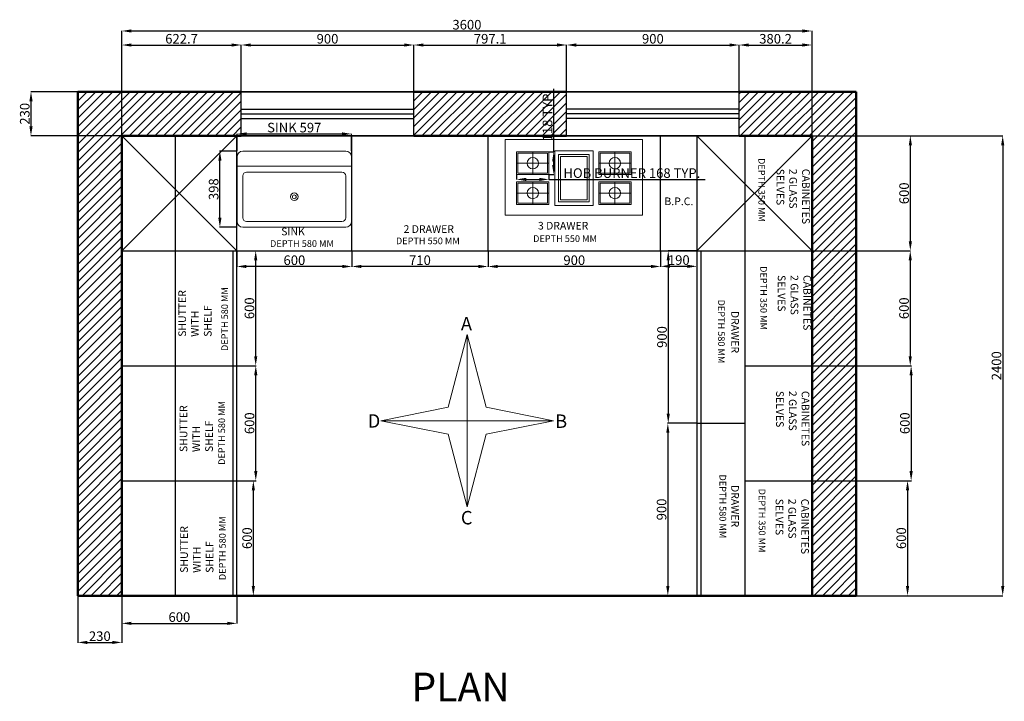
# Model space of a CAD drawing. Units: millimetres. Extents: x 4283 to 9420, y -2853 to 5191.
# Tile 2 of 2: x 4283 to 9420, y 1633 to 5191. Entities that reach past the tile are written whole.
import ezdxf

# ---------------------------------------------------------------- set-up
doc = ezdxf.new("R2010")
doc.units = ezdxf.units.MM
for name, color, linetype, lineweight in [('A-ANNO-DIMS', 2, 'Continuous', 18), ('A-ANNO-SYMB', 7, 'Continuous', 18), ('A-ANNO-TEXT', 7, 'Continuous', 18), ('A-EQPM', 8, 'Continuous', 18), ('A-FLOR-FIXT', 8, 'Continuous', 18), ('A-FURN', 3, 'Continuous', 25), ('A-GLAZ', 4, 'Continuous', 25), ('A-WALL', 24, 'Continuous', 50), ('A-WALL-PATT', 32, 'Continuous', 13)]:
    doc.layers.add(name, color=color, linetype=linetype, lineweight=lineweight)
doc.styles.get("Standard").update_dxf_attribs({"font": 'arial.ttf'})
doc.dimstyles.new('ISO-25', dxfattribs={"dimtxt": 50, "dimasz": 50, "dimexe": 1.25, "dimexo": 0.625, "dimtad": 1, "dimdec": 0, "dimtxsty": 'Standard', "dimcen": 2.5, "dimclrd": 4, "dimclre": 4, "dimclrt": 4, "dimadec": 0, "dimazin": 0, "dimtfac": 1, "dimtdec": 0, "dimtmove": 0, "dimatfit": 3, "dimfxl": 1, "dimarcsym": 0})

# ---------------------------------------------------------------- blocks, each defined once
blk = doc.blocks.new('Sink-single - 30 in top')
blk.add_line((-15, -3.999996), (15, -3.999996))
for points in [[(-13.5, 0), (13.5, 0)], [(-15, -18.499996), (-15, -1.5)], [(15, -1.5), (15, -18.499996)], [(-13.5, -17.499996), (-13.5, -6.499996)], [(-12.5, -5.499996), (12.5, -5.499996)], [(13.5, -6.499996), (13.5, -17.499996)], [(13.5, -19.999996), (-13.5, -19.999996)], [(12.5, -18.499996), (-12.5, -18.499996)]]:
    blk.add_lwpolyline(points)
for radius in [1, 0.5]:
    blk.add_circle((0, -11.999996), radius)
for centre, radius, start, end in [((-13.5, -1.5), 1.5, 90, 180), ((13.5, -1.5), 1.5, 0, 90), ((-12.5, -6.499996), 1, 90, 180), ((12.5, -6.499996), 1, 0, 90), ((-12.5, -17.499996), 1, 180, 270), ((12.5, -17.499996), 1, 270, 0), ((-13.5, -18.499996), 1.5, 180, 270), ((13.5, -18.499996), 1.5, 270, 0)]:
    blk.add_arc(centre, radius, start, end)
blk = doc.blocks.new('*D4')
at = {"layer": 'A-ANNO-DIMS', "color": 0, "lineweight": -2, "transparency": 16777216}
for p, q in [((4816.4, 4585.1), (4816.4, 5133)), ((4866.4, 5131.7), (8366.4, 5131.7)), ((8416.4, 4585.1), (8416.4, 5133))]:
    blk.add_line(p, q, dxfattribs=at)
at = {"layer": 'A-ANNO-DIMS', "color": 0, "transparency": 16777216}
for points in [[(4866.4, 5140), (4866.4, 5123.4), (4816.4, 5131.7)], [(8366.4, 5140), (8366.4, 5123.4), (8416.4, 5131.7)]]:
    blk.add_solid(points, dxfattribs=at)
at = {"layer": 'Defpoints', "color": 0, "transparency": 16777216}
for p in [(8416.4, 5131.7), (4816.4, 4584.5), (8416.4, 4584.5)]:
    blk.add_point(p, dxfattribs=at)
at = {"layer": 'A-ANNO-DIMS', "color": 0, "transparency": 16777216, "insert": (6616.4, 5157.9), "char_height": 50, "attachment_point": 5}
blk.add_mtext('3600', dxfattribs=at)
blk = doc.blocks.new('*D5')
at = {"layer": 'A-ANNO-DIMS', "color": 0, "lineweight": -2, "transparency": 16777216}
for p, q in [((8417.1, 4584.5), (9412.4, 4584.5)), ((9411.2, 4534.5), (9411.2, 2234.5)), ((8417.1, 2184.5), (9412.4, 2184.5))]:
    blk.add_line(p, q, dxfattribs=at)
at = {"layer": 'A-ANNO-DIMS', "color": 0, "transparency": 16777216}
for points in [[(9402.8, 4534.5), (9419.5, 4534.5), (9411.2, 4584.5)], [(9402.8, 2234.5), (9419.5, 2234.5), (9411.2, 2184.5)]]:
    blk.add_solid(points, dxfattribs=at)
at = {"layer": 'Defpoints', "color": 0, "transparency": 16777216}
for p in [(8416.4, 4584.5), (8416.4, 2184.5), (9411.2, 2184.5)]:
    blk.add_point(p, dxfattribs=at)
at = {"layer": 'A-ANNO-DIMS', "color": 0, "transparency": 16777216, "insert": (9385, 3384.5), "char_height": 50, "attachment_point": 5, "rotation": 90}
blk.add_mtext('2400', dxfattribs=at)
blk = doc.blocks.new('*D6')
at = {"layer": 'A-ANNO-DIMS', "color": 0, "lineweight": -2, "transparency": 16777216}
for p, q in [((8417.1, 4584.5), (8930.6, 4584.5)), ((8929.3, 4534.5), (8929.3, 4034.5)), ((8417.1, 3984.5), (8930.6, 3984.5))]:
    blk.add_line(p, q, dxfattribs=at)
at = {"layer": 'A-ANNO-DIMS', "color": 0, "transparency": 16777216}
for points in [[(8921, 4534.5), (8937.7, 4534.5), (8929.3, 4584.5)], [(8921, 4034.5), (8937.7, 4034.5), (8929.3, 3984.5)]]:
    blk.add_solid(points, dxfattribs=at)
at = {"layer": 'Defpoints', "color": 0, "transparency": 16777216}
for p in [(8416.4, 4584.5), (8416.4, 3984.5), (8929.3, 3984.5)]:
    blk.add_point(p, dxfattribs=at)
at = {"layer": 'A-ANNO-DIMS', "color": 0, "transparency": 16777216, "insert": (8903.2, 4284.5), "char_height": 50, "attachment_point": 5, "rotation": 90}
blk.add_mtext('600', dxfattribs=at)
blk = doc.blocks.new('*D7')
at = {"layer": 'A-ANNO-DIMS', "color": 0, "lineweight": -2, "transparency": 16777216}
for p, q in [((8417.1, 3984.5), (8930.2, 3984.5)), ((8928.9, 3934.5), (8928.9, 3434.5)), ((8417.1, 3384.5), (8930.2, 3384.5))]:
    blk.add_line(p, q, dxfattribs=at)
at = {"layer": 'A-ANNO-DIMS', "color": 0, "transparency": 16777216}
for points in [[(8920.6, 3934.5), (8937.3, 3934.5), (8928.9, 3984.5)], [(8920.6, 3434.5), (8937.3, 3434.5), (8928.9, 3384.5)]]:
    blk.add_solid(points, dxfattribs=at)
at = {"layer": 'Defpoints', "color": 0, "transparency": 16777216}
for p in [(8416.4, 3984.5), (8416.4, 3384.5), (8928.9, 3384.5)]:
    blk.add_point(p, dxfattribs=at)
at = {"layer": 'A-ANNO-DIMS', "color": 0, "transparency": 16777216, "insert": (8902.8, 3684.5), "char_height": 50, "attachment_point": 5, "rotation": 90}
blk.add_mtext('600', dxfattribs=at)
blk = doc.blocks.new('*D8')
at = {"layer": 'A-ANNO-DIMS', "color": 0, "lineweight": -2, "transparency": 16777216}
for p, q in [((8067.1, 3384.5), (8934.8, 3384.5)), ((8933.5, 3334.5), (8933.5, 2834.5)), ((8067.1, 2784.5), (8934.8, 2784.5))]:
    blk.add_line(p, q, dxfattribs=at)
at = {"layer": 'A-ANNO-DIMS', "color": 0, "transparency": 16777216}
for points in [[(8925.2, 3334.5), (8941.9, 3334.5), (8933.5, 3384.5)], [(8925.2, 2834.5), (8941.9, 2834.5), (8933.5, 2784.5)]]:
    blk.add_solid(points, dxfattribs=at)
at = {"layer": 'Defpoints', "color": 0, "transparency": 16777216}
for p in [(8066.4, 3384.5), (8066.4, 2784.5), (8933.5, 2784.5)]:
    blk.add_point(p, dxfattribs=at)
at = {"layer": 'A-ANNO-DIMS', "color": 0, "transparency": 16777216, "insert": (8907.4, 3084.5), "char_height": 50, "attachment_point": 5, "rotation": 90}
blk.add_mtext('600', dxfattribs=at)
blk = doc.blocks.new('*D9')
at = {"layer": 'A-ANNO-DIMS', "color": 0, "lineweight": -2, "transparency": 16777216}
for p, q in [((8067.1, 2784.5), (8916, 2784.5)), ((8914.7, 2734.5), (8914.7, 2234.5)), ((8067.1, 2184.5), (8916, 2184.5))]:
    blk.add_line(p, q, dxfattribs=at)
at = {"layer": 'A-ANNO-DIMS', "color": 0, "transparency": 16777216}
for points in [[(8906.4, 2734.5), (8923.1, 2734.5), (8914.7, 2784.5)], [(8906.4, 2234.5), (8923.1, 2234.5), (8914.7, 2184.5)]]:
    blk.add_solid(points, dxfattribs=at)
at = {"layer": 'Defpoints', "color": 0, "transparency": 16777216}
for p in [(8066.4, 2784.5), (8066.4, 2184.5), (8914.7, 2184.5)]:
    blk.add_point(p, dxfattribs=at)
at = {"layer": 'A-ANNO-DIMS', "color": 0, "transparency": 16777216, "insert": (8888.6, 2484.5), "char_height": 50, "attachment_point": 5, "rotation": 90}
blk.add_mtext('600', dxfattribs=at)
blk = doc.blocks.new('*D10')
at = {"layer": 'A-ANNO-DIMS', "color": 0, "lineweight": -2, "transparency": 16777216}
for p, q in [((7815.8, 3984.5), (7665.3, 3984.5)), ((7666.5, 3934.5), (7666.5, 3134.5)), ((7815.8, 3084.5), (7665.3, 3084.5))]:
    blk.add_line(p, q, dxfattribs=at)
at = {"layer": 'A-ANNO-DIMS', "color": 0, "transparency": 16777216}
for points in [[(7658.2, 3934.5), (7674.8, 3934.5), (7666.5, 3984.5)], [(7658.2, 3134.5), (7674.8, 3134.5), (7666.5, 3084.5)]]:
    blk.add_solid(points, dxfattribs=at)
at = {"layer": 'Defpoints', "color": 0, "transparency": 16777216}
for p in [(7816.4, 3984.5), (7666.5, 3084.5), (7816.4, 3084.5)]:
    blk.add_point(p, dxfattribs=at)
at = {"layer": 'A-ANNO-DIMS', "color": 0, "transparency": 16777216, "insert": (7640.4, 3534.5), "char_height": 50, "attachment_point": 5, "rotation": 90}
blk.add_mtext('900', dxfattribs=at)
blk = doc.blocks.new('*D11')
at = {"layer": 'A-ANNO-DIMS', "color": 0, "lineweight": -2, "transparency": 16777216}
for p, q in [((7815.8, 3084.5), (7663.2, 3084.5)), ((7664.4, 3034.5), (7664.4, 2234.5)), ((7815.8, 2184.5), (7663.2, 2184.5))]:
    blk.add_line(p, q, dxfattribs=at)
at = {"layer": 'A-ANNO-DIMS', "color": 0, "transparency": 16777216}
for points in [[(7656.1, 3034.5), (7672.7, 3034.5), (7664.4, 3084.5)], [(7656.1, 2234.5), (7672.7, 2234.5), (7664.4, 2184.5)]]:
    blk.add_solid(points, dxfattribs=at)
at = {"layer": 'Defpoints', "color": 0, "transparency": 16777216}
for p in [(7816.4, 3084.5), (7664.4, 2184.5), (7816.4, 2184.5)]:
    blk.add_point(p, dxfattribs=at)
at = {"layer": 'A-ANNO-DIMS', "color": 0, "transparency": 16777216, "insert": (7638.3, 2634.5), "char_height": 50, "attachment_point": 5, "rotation": 90}
blk.add_mtext('900', dxfattribs=at)
blk = doc.blocks.new('*D12')
at = {"layer": 'A-ANNO-DIMS', "color": 0, "lineweight": -2, "transparency": 16777216}
for p, q in [((7626.4, 3983.8), (7626.4, 3902.2)), ((7816.4, 3983.8), (7816.4, 3902.2)), ((7676.4, 3903.4), (7766.4, 3903.4))]:
    blk.add_line(p, q, dxfattribs=at)
at = {"layer": 'A-ANNO-DIMS', "color": 0, "transparency": 16777216}
for points in [[(7676.4, 3911.8), (7676.4, 3895.1), (7626.4, 3903.4)], [(7766.4, 3911.8), (7766.4, 3895.1), (7816.4, 3903.4)]]:
    blk.add_solid(points, dxfattribs=at)
at = {"layer": 'Defpoints', "color": 0, "transparency": 16777216}
for p in [(7626.4, 3984.5), (7816.4, 3984.5), (7816.4, 3903.4)]:
    blk.add_point(p, dxfattribs=at)
at = {"layer": 'A-ANNO-DIMS', "color": 0, "transparency": 16777216, "insert": (7721.4, 3929.6), "char_height": 50, "attachment_point": 5}
blk.add_mtext('190', dxfattribs=at)
blk = doc.blocks.new('*D13')
at = {"layer": 'A-ANNO-DIMS', "color": 0, "lineweight": -2, "transparency": 16777216}
for p, q in [((6726.4, 3983.8), (6726.4, 3901.4)), ((7626.4, 3983.8), (7626.4, 3901.4)), ((7576.4, 3902.6), (6776.4, 3902.6))]:
    blk.add_line(p, q, dxfattribs=at)
at = {"layer": 'A-ANNO-DIMS', "color": 0, "transparency": 16777216}
for points in [[(6776.4, 3911), (6776.4, 3894.3), (6726.4, 3902.6)], [(7576.4, 3911), (7576.4, 3894.3), (7626.4, 3902.6)]]:
    blk.add_solid(points, dxfattribs=at)
at = {"layer": 'Defpoints', "color": 0, "transparency": 16777216}
for p in [(6726.4, 3984.5), (7626.4, 3984.5), (6726.4, 3902.6)]:
    blk.add_point(p, dxfattribs=at)
at = {"layer": 'A-ANNO-DIMS', "color": 0, "transparency": 16777216, "insert": (7176.4, 3928.8), "char_height": 50, "attachment_point": 5}
blk.add_mtext('900', dxfattribs=at)
blk = doc.blocks.new('*D14')
at = {"layer": 'A-ANNO-DIMS', "color": 0, "lineweight": -2, "transparency": 16777216}
for p, q in [((6016.4, 3983.8), (6016.4, 3901.4)), ((6726.4, 3983.8), (6726.4, 3901.4)), ((6676.4, 3902.6), (6066.4, 3902.6))]:
    blk.add_line(p, q, dxfattribs=at)
at = {"layer": 'A-ANNO-DIMS', "color": 0, "transparency": 16777216}
for points in [[(6066.4, 3911), (6066.4, 3894.3), (6016.4, 3902.6)], [(6676.4, 3911), (6676.4, 3894.3), (6726.4, 3902.6)]]:
    blk.add_solid(points, dxfattribs=at)
at = {"layer": 'Defpoints', "color": 0, "transparency": 16777216}
for p in [(6016.4, 3984.5), (6726.4, 3984.5), (6016.4, 3902.6)]:
    blk.add_point(p, dxfattribs=at)
at = {"layer": 'A-ANNO-DIMS', "color": 0, "transparency": 16777216, "insert": (6371.4, 3928.8), "char_height": 50, "attachment_point": 5}
blk.add_mtext('710', dxfattribs=at)
blk = doc.blocks.new('*D15')
at = {"layer": 'A-ANNO-DIMS', "color": 0, "lineweight": -2, "transparency": 16777216}
for p, q in [((5416.4, 3983.8), (5416.4, 3901.4)), ((6016.4, 3983.8), (6016.4, 3901.4)), ((5966.4, 3902.6), (5466.4, 3902.6))]:
    blk.add_line(p, q, dxfattribs=at)
at = {"layer": 'A-ANNO-DIMS', "color": 0, "transparency": 16777216}
for points in [[(5466.4, 3911), (5466.4, 3894.3), (5416.4, 3902.6)], [(5966.4, 3911), (5966.4, 3894.3), (6016.4, 3902.6)]]:
    blk.add_solid(points, dxfattribs=at)
at = {"layer": 'Defpoints', "color": 0, "transparency": 16777216}
for p in [(5416.4, 3984.5), (6016.4, 3984.5), (5416.4, 3902.6)]:
    blk.add_point(p, dxfattribs=at)
at = {"layer": 'A-ANNO-DIMS', "color": 0, "transparency": 16777216, "insert": (5716.4, 3928.8), "char_height": 50, "attachment_point": 5}
blk.add_mtext('600', dxfattribs=at)
blk = doc.blocks.new('*D16')
at = {"layer": 'A-ANNO-DIMS', "color": 0, "lineweight": -2, "transparency": 16777216}
for p, q in [((5417.1, 2784.5), (5503.6, 2784.5)), ((5502.3, 2234.5), (5502.3, 2734.5)), ((5417.1, 2184.5), (5503.6, 2184.5))]:
    blk.add_line(p, q, dxfattribs=at)
at = {"layer": 'A-ANNO-DIMS', "color": 0, "transparency": 16777216}
for points in [[(5494, 2734.5), (5510.6, 2734.5), (5502.3, 2784.5)], [(5494, 2234.5), (5510.6, 2234.5), (5502.3, 2184.5)]]:
    blk.add_solid(points, dxfattribs=at)
at = {"layer": 'Defpoints', "color": 0, "transparency": 16777216}
for p in [(5416.4, 2784.5), (5502.3, 2784.5), (5416.4, 2184.5)]:
    blk.add_point(p, dxfattribs=at)
at = {"layer": 'A-ANNO-DIMS', "color": 0, "transparency": 16777216, "insert": (5476.2, 2484.5), "char_height": 50, "attachment_point": 5, "rotation": 90}
blk.add_mtext('600', dxfattribs=at)
blk = doc.blocks.new('*D17')
at = {"layer": 'A-ANNO-DIMS', "color": 0, "lineweight": -2, "transparency": 16777216}
for p, q in [((5417.1, 3384.5), (5516.2, 3384.5)), ((5514.9, 2834.5), (5514.9, 3334.5)), ((5417.1, 2784.5), (5516.2, 2784.5))]:
    blk.add_line(p, q, dxfattribs=at)
at = {"layer": 'A-ANNO-DIMS', "color": 0, "transparency": 16777216}
for points in [[(5506.6, 3334.5), (5523.3, 3334.5), (5514.9, 3384.5)], [(5506.6, 2834.5), (5523.3, 2834.5), (5514.9, 2784.5)]]:
    blk.add_solid(points, dxfattribs=at)
at = {"layer": 'Defpoints', "color": 0, "transparency": 16777216}
for p in [(5416.4, 3384.5), (5514.9, 3384.5), (5416.4, 2784.5)]:
    blk.add_point(p, dxfattribs=at)
at = {"layer": 'A-ANNO-DIMS', "color": 0, "transparency": 16777216, "insert": (5488.8, 3084.5), "char_height": 50, "attachment_point": 5, "rotation": 90}
blk.add_mtext('600', dxfattribs=at)
blk = doc.blocks.new('*D18')
at = {"layer": 'A-ANNO-DIMS', "color": 0, "lineweight": -2, "transparency": 16777216}
for p, q in [((5417.1, 3984.5), (5515.8, 3984.5)), ((5514.6, 3434.5), (5514.6, 3934.5)), ((5417.1, 3384.5), (5515.8, 3384.5))]:
    blk.add_line(p, q, dxfattribs=at)
at = {"layer": 'A-ANNO-DIMS', "color": 0, "transparency": 16777216}
for points in [[(5506.3, 3934.5), (5522.9, 3934.5), (5514.6, 3984.5)], [(5506.3, 3434.5), (5522.9, 3434.5), (5514.6, 3384.5)]]:
    blk.add_solid(points, dxfattribs=at)
at = {"layer": 'Defpoints', "color": 0, "transparency": 16777216}
for p in [(5416.4, 3984.5), (5514.6, 3984.5), (5416.4, 3384.5)]:
    blk.add_point(p, dxfattribs=at)
at = {"layer": 'A-ANNO-DIMS', "color": 0, "transparency": 16777216, "insert": (5488.4, 3684.5), "char_height": 50, "attachment_point": 5, "rotation": 90}
blk.add_mtext('600', dxfattribs=at)
blk = doc.blocks.new('*D19')
at = {"layer": 'A-ANNO-DIMS', "color": 0, "lineweight": -2, "transparency": 16777216}
for p, q in [((4816.4, 2183.8), (4816.4, 2038.8)), ((5416.4, 2183.8), (5416.4, 2038.8)), ((4866.4, 2040), (5366.4, 2040))]:
    blk.add_line(p, q, dxfattribs=at)
at = {"layer": 'A-ANNO-DIMS', "color": 0, "transparency": 16777216}
for points in [[(4866.4, 2048.3), (4866.4, 2031.7), (4816.4, 2040)], [(5366.4, 2048.3), (5366.4, 2031.7), (5416.4, 2040)]]:
    blk.add_solid(points, dxfattribs=at)
at = {"layer": 'Defpoints', "color": 0, "transparency": 16777216}
for p in [(4816.4, 2184.5), (5416.4, 2184.5), (5416.4, 2040)]:
    blk.add_point(p, dxfattribs=at)
at = {"layer": 'A-ANNO-DIMS', "color": 0, "transparency": 16777216, "insert": (5116.4, 2066.2), "char_height": 50, "attachment_point": 5}
blk.add_mtext('600', dxfattribs=at)
blk = doc.blocks.new('HOB-BURNER')
for p, q in [((6959.7, 4500.7), (6959.7, 4382.2)), ((6875.6, 4441.4), (7043.8, 4441.4))]:
    blk.add_line(p, q)
for points in [[(7043.8, 4500.7), (6875.6, 4500.7), (6875.6, 4382.2), (7043.8, 4382.2)], [(7036.8, 4493.7), (6882.6, 4493.7), (6882.6, 4389.2), (7036.8, 4389.2)]]:
    blk.add_lwpolyline(points, close=True)
blk.add_circle((6959.7, 4441.4), 29.8)
blk = doc.blocks.new('*D39')
at = {"layer": 'A-ANNO-DIMS', "color": 4, "lineweight": -2, "transparency": 16777216}
for p, q in [((6875.6, 4381.6), (6875.6, 4355.8)), ((7043.8, 4381.6), (7043.8, 4355.8)), ((6925.6, 4357), (6993.8, 4357)), ((7043.8, 4357), (7859.7, 4357))]:
    blk.add_line(p, q, dxfattribs=at)
at = {"layer": 'A-ANNO-DIMS', "color": 4, "transparency": 16777216}
for points in [[(6925.6, 4365.3), (6925.6, 4348.7), (6875.6, 4357)], [(6993.8, 4365.3), (6993.8, 4348.7), (7043.8, 4357)]]:
    blk.add_solid(points, dxfattribs=at)
at = {"layer": 'Defpoints', "color": 0, "transparency": 16777216}
for p in [(6875.6, 4382.2), (7043.8, 4382.2), (7043.8, 4357)]:
    blk.add_point(p, dxfattribs=at)
at = {"layer": 'A-ANNO-DIMS', "color": 4, "transparency": 16777216, "insert": (7476.7, 4383.5), "char_height": 50, "attachment_point": 5}
blk.add_mtext('HOB BURNER 168 TYP.', dxfattribs=at)
blk = doc.blocks.new('*D40')
at = {"layer": 'A-ANNO-DIMS', "color": 4, "lineweight": -2, "transparency": 16777216}
for p, q in [((7069, 4500.7), (7069, 4829.4)), ((7044.4, 4500.7), (7070.3, 4500.7)), ((7069, 4432.2), (7069, 4450.7)), ((7044.4, 4382.2), (7070.3, 4382.2))]:
    blk.add_line(p, q, dxfattribs=at)
at = {"layer": 'A-ANNO-DIMS', "color": 4, "transparency": 16777216}
for points in [[(7060.7, 4450.7), (7077.3, 4450.7), (7069, 4500.7)], [(7060.7, 4432.2), (7077.3, 4432.2), (7069, 4382.2)]]:
    blk.add_solid(points, dxfattribs=at)
at = {"layer": 'Defpoints', "color": 0, "transparency": 16777216}
for p in [(7043.8, 4500.7), (7069, 4500.7), (7043.8, 4382.2)]:
    blk.add_point(p, dxfattribs=at)
at = {"layer": 'A-ANNO-DIMS', "color": 4, "transparency": 16777216, "insert": (7042.9, 4690), "char_height": 50, "attachment_point": 5, "rotation": 90}
blk.add_mtext('118 TYP.', dxfattribs=at)
blk = doc.blocks.new('*D41')
at = {"layer": 'A-ANNO-DIMS', "color": 4, "lineweight": -2, "transparency": 16777216}
for p, q in [((5417.3, 4505.5), (5417.3, 4595.7)), ((5467.3, 4594.4), (5964, 4594.4)), ((6014, 4505.5), (6014, 4595.7))]:
    blk.add_line(p, q, dxfattribs=at)
at = {"layer": 'A-ANNO-DIMS', "color": 4, "transparency": 16777216}
for points in [[(5467.3, 4602.8), (5467.3, 4586.1), (5417.3, 4594.4)], [(5964, 4602.8), (5964, 4586.1), (6014, 4594.4)]]:
    blk.add_solid(points, dxfattribs=at)
at = {"layer": 'Defpoints', "color": 0, "transparency": 16777216}
for p in [(6014, 4594.4), (5417.3, 4504.9), (6014, 4504.9)]:
    blk.add_point(p, dxfattribs=at)
at = {"layer": 'A-ANNO-DIMS', "color": 4, "transparency": 16777216, "insert": (5715.7, 4620.9), "char_height": 50, "attachment_point": 5}
blk.add_mtext('SINK 597', dxfattribs=at)
blk = doc.blocks.new('*D42')
at = {"layer": 'A-ANNO-DIMS', "color": 4, "lineweight": -2, "transparency": 16777216}
for p, q in [((5416.7, 4504.9), (5326.5, 4504.9)), ((5327.8, 4157.1), (5327.8, 4454.9)), ((5416.7, 4107.1), (5326.5, 4107.1))]:
    blk.add_line(p, q, dxfattribs=at)
at = {"layer": 'A-ANNO-DIMS', "color": 4, "transparency": 16777216}
for points in [[(5319.5, 4454.9), (5336.1, 4454.9), (5327.8, 4504.9)], [(5319.5, 4157.1), (5336.1, 4157.1), (5327.8, 4107.1)]]:
    blk.add_solid(points, dxfattribs=at)
at = {"layer": 'Defpoints', "color": 0, "transparency": 16777216}
for p in [(5327.8, 4504.9), (5417.3, 4504.9), (5417.3, 4107.1)]:
    blk.add_point(p, dxfattribs=at)
at = {"layer": 'A-ANNO-DIMS', "color": 4, "transparency": 16777216, "insert": (5301.6, 4306), "char_height": 50, "attachment_point": 5, "rotation": 90}
blk.add_mtext('398', dxfattribs=at)
blk = doc.blocks.new('*D43')
at = {"layer": 'A-ANNO-DIMS', "color": 4, "lineweight": -2, "transparency": 16777216}
for p, q in [((4586.4, 2183.8), (4586.4, 1939.2)), ((4816.4, 2183.8), (4816.4, 1939.2)), ((4636.4, 1940.5), (4766.4, 1940.5))]:
    blk.add_line(p, q, dxfattribs=at)
at = {"layer": 'A-ANNO-DIMS', "color": 4, "transparency": 16777216}
for points in [[(4636.4, 1948.8), (4636.4, 1932.1), (4586.4, 1940.5)], [(4766.4, 1948.8), (4766.4, 1932.1), (4816.4, 1940.5)]]:
    blk.add_solid(points, dxfattribs=at)
at = {"layer": 'Defpoints', "color": 0, "transparency": 16777216}
for p in [(4586.4, 2184.5), (4816.4, 2184.5), (4816.4, 1940.5)]:
    blk.add_point(p, dxfattribs=at)
at = {"layer": 'A-ANNO-DIMS', "color": 4, "transparency": 16777216, "insert": (4701.4, 1966.6), "char_height": 50, "attachment_point": 5}
blk.add_mtext('230', dxfattribs=at)
blk = doc.blocks.new('*D44')
at = {"layer": 'A-ANNO-DIMS', "color": 4, "lineweight": -2, "transparency": 16777216}
for p, q in [((8035.6, 4814.5), (4341.2, 4814.5)), ((4342.4, 4764.5), (4342.4, 4634.5)), ((8035.6, 4584.5), (4341.2, 4584.5))]:
    blk.add_line(p, q, dxfattribs=at)
at = {"layer": 'A-ANNO-DIMS', "color": 4, "transparency": 16777216}
for points in [[(4334.1, 4764.5), (4350.8, 4764.5), (4342.4, 4814.5)], [(4334.1, 4634.5), (4350.8, 4634.5), (4342.4, 4584.5)]]:
    blk.add_solid(points, dxfattribs=at)
at = {"layer": 'Defpoints', "color": 0, "transparency": 16777216}
for p in [(8036.3, 4814.5), (4342.4, 4584.5), (8036.3, 4584.5)]:
    blk.add_point(p, dxfattribs=at)
at = {"layer": 'A-ANNO-DIMS', "color": 4, "transparency": 16777216, "insert": (4316.3, 4699.5), "char_height": 50, "attachment_point": 5, "rotation": 90}
blk.add_mtext('230', dxfattribs=at)
blk = doc.blocks.new('*D45')
at = {"layer": 'A-ANNO-DIMS', "color": 4, "lineweight": -2, "transparency": 16777216}
for p, q in [((4816.4, 4585.1), (4816.4, 5059.7)), ((4866.4, 5058.5), (5389.1, 5058.5)), ((5439.1, 4585.1), (5439.1, 5059.7))]:
    blk.add_line(p, q, dxfattribs=at)
at = {"layer": 'A-ANNO-DIMS', "color": 4, "transparency": 16777216}
for points in [[(4866.4, 5066.8), (4866.4, 5050.1), (4816.4, 5058.5)], [(5389.1, 5066.8), (5389.1, 5050.1), (5439.1, 5058.5)]]:
    blk.add_solid(points, dxfattribs=at)
at = {"layer": 'Defpoints', "color": 0, "transparency": 16777216}
for p in [(5439.1, 5058.5), (4816.4, 4584.5), (5439.1, 4584.5)]:
    blk.add_point(p, dxfattribs=at)
at = {"layer": 'A-ANNO-DIMS', "color": 4, "transparency": 16777216, "insert": (5127.8, 5084.6), "char_height": 50, "attachment_point": 5}
blk.add_mtext('622.7', dxfattribs=at)
blk = doc.blocks.new('*D46')
at = {"layer": 'A-ANNO-DIMS', "color": 4, "lineweight": -2, "transparency": 16777216}
for p, q in [((5439.1, 4585.1), (5439.1, 5059.7)), ((5489.1, 5058.5), (6289.1, 5058.5)), ((6339.1, 4585.1), (6339.1, 5059.7))]:
    blk.add_line(p, q, dxfattribs=at)
at = {"layer": 'A-ANNO-DIMS', "color": 4, "transparency": 16777216}
for points in [[(5489.1, 5066.8), (5489.1, 5050.1), (5439.1, 5058.5)], [(6289.1, 5066.8), (6289.1, 5050.1), (6339.1, 5058.5)]]:
    blk.add_solid(points, dxfattribs=at)
at = {"layer": 'Defpoints', "color": 0, "transparency": 16777216}
for p in [(6339.1, 5058.5), (5439.1, 4584.5), (6339.1, 4584.5)]:
    blk.add_point(p, dxfattribs=at)
at = {"layer": 'A-ANNO-DIMS', "color": 4, "transparency": 16777216, "insert": (5889.1, 5084.6), "char_height": 50, "attachment_point": 5}
blk.add_mtext('900', dxfattribs=at)
blk = doc.blocks.new('*D47')
at = {"layer": 'A-ANNO-DIMS', "color": 4, "lineweight": -2, "transparency": 16777216}
for p, q in [((6339.1, 4585.1), (6339.1, 5059.7)), ((6389.1, 5058.5), (7086.3, 5058.5)), ((7136.3, 4585.1), (7136.3, 5059.7))]:
    blk.add_line(p, q, dxfattribs=at)
at = {"layer": 'A-ANNO-DIMS', "color": 4, "transparency": 16777216}
for points in [[(6389.1, 5066.8), (6389.1, 5050.1), (6339.1, 5058.5)], [(7086.3, 5066.8), (7086.3, 5050.1), (7136.3, 5058.5)]]:
    blk.add_solid(points, dxfattribs=at)
at = {"layer": 'Defpoints', "color": 0, "transparency": 16777216}
for p in [(7136.3, 5058.5), (6339.1, 4584.5), (7136.3, 4584.5)]:
    blk.add_point(p, dxfattribs=at)
at = {"layer": 'A-ANNO-DIMS', "color": 4, "transparency": 16777216, "insert": (6737.7, 5084.6), "char_height": 50, "attachment_point": 5}
blk.add_mtext('797.1', dxfattribs=at)
blk = doc.blocks.new('*D48')
at = {"layer": 'A-ANNO-DIMS', "color": 4, "lineweight": -2, "transparency": 16777216}
for p, q in [((7136.3, 4585.1), (7136.3, 5059.7)), ((7186.3, 5058.5), (7986.3, 5058.5)), ((8036.3, 4585.1), (8036.3, 5059.7))]:
    blk.add_line(p, q, dxfattribs=at)
at = {"layer": 'A-ANNO-DIMS', "color": 4, "transparency": 16777216}
for points in [[(7186.3, 5066.8), (7186.3, 5050.1), (7136.3, 5058.5)], [(7986.3, 5066.8), (7986.3, 5050.1), (8036.3, 5058.5)]]:
    blk.add_solid(points, dxfattribs=at)
at = {"layer": 'Defpoints', "color": 0, "transparency": 16777216}
for p in [(8036.3, 5058.5), (7136.3, 4584.5), (8036.3, 4584.5)]:
    blk.add_point(p, dxfattribs=at)
at = {"layer": 'A-ANNO-DIMS', "color": 4, "transparency": 16777216, "insert": (7586.3, 5084.6), "char_height": 50, "attachment_point": 5}
blk.add_mtext('900', dxfattribs=at)
blk = doc.blocks.new('*D49')
at = {"layer": 'A-ANNO-DIMS', "color": 4, "lineweight": -2, "transparency": 16777216}
for p, q in [((8036.3, 4585.1), (8036.3, 5059.7)), ((8086.3, 5058.5), (8366.4, 5058.5)), ((8416.4, 4585.1), (8416.4, 5059.7))]:
    blk.add_line(p, q, dxfattribs=at)
at = {"layer": 'A-ANNO-DIMS', "color": 4, "transparency": 16777216}
for points in [[(8086.3, 5066.8), (8086.3, 5050.1), (8036.3, 5058.5)], [(8366.4, 5066.8), (8366.4, 5050.1), (8416.4, 5058.5)]]:
    blk.add_solid(points, dxfattribs=at)
at = {"layer": 'Defpoints', "color": 0, "transparency": 16777216}
for p in [(8416.4, 5058.5), (8036.3, 4584.5), (8416.4, 4584.5)]:
    blk.add_point(p, dxfattribs=at)
at = {"layer": 'A-ANNO-DIMS', "color": 4, "transparency": 16777216, "insert": (8226.3, 5084.6), "char_height": 50, "attachment_point": 5}
blk.add_mtext('380.2', dxfattribs=at)

msp = doc.modelspace()

# ---------------------------------------------------------------- hatches: boundary and pattern name
at = {"layer": 'A-WALL-PATT'}
h = msp.add_hatch(dxfattribs=at)
h.set_pattern_fill('ANSI31', color=256, scale=10)
h.paths.add_polyline_path([(4816.43, 4584.47), (5439.12, 4584.47), (5439.12, 4814.47), (4586.43, 4814.47), (4586.43, 2184.47), (4816.43, 2184.47)])
h.paths.add_polyline_path([(6339.12, 4814.47), (6339.12, 4584.47), (7136.26, 4584.47), (7136.26, 4814.47)])
h.paths.add_polyline_path([(8646.43, 4814.47), (8036.26, 4814.47), (8036.26, 4584.47), (8416.43, 4584.47), (8416.43, 2184.47), (8646.43, 2184.47)])

# ---------------------------------------------------------------- linework, layer by layer
at = {"layer": 'A-ANNO-SYMB'}
for p, q in [((6617.95, 3547.65), (6518.8, 3167.65)), ((6617.95, 3547.65), (6617.95, 2647.65)), ((6617.95, 3547.65), (6717.11, 3167.65)), ((6518.8, 3167.65), (6167.95, 3097.65)), ((6717.11, 3167.65), (7067.95, 3097.65)), ((6167.95, 3097.65), (6617.95, 3097.65)), ((6518.8, 3027.65), (6167.95, 3097.65)), ((6617.95, 3097.65), (7067.95, 3097.65)), ((6717.11, 3027.65), (7067.95, 3097.65)), ((6617.95, 2647.65), (6518.8, 3027.65)), ((6617.95, 2647.65), (6717.11, 3027.65))]:
    msp.add_line(p, q, dxfattribs=at)
at = {"layer": 'A-EQPM'}
for p, q in [((7074.05, 4506.82), (7074.05, 4220.35)), ((7274.05, 4506.82), (7274.05, 4220.35))]:
    msp.add_line(p, q, dxfattribs=at)
for points in [[(6815.51, 4564.47), (7532.58, 4564.47), (7532.58, 4170.57), (6815.51, 4170.57)], [(7074.05, 4506.82), (7274.05, 4506.82), (7274.05, 4220.35), (7074.05, 4220.35)], [(7094.05, 4486.82), (7254.05, 4486.82), (7254.05, 4240.35), (7094.05, 4240.35)], [(7104.05, 4476.82), (7244.05, 4476.82), (7244.05, 4250.35), (7104.05, 4250.35)]]:
    msp.add_lwpolyline(points, close=True, dxfattribs=at)
at = {"layer": 'A-FURN'}
for p, q in [((4816.43, 3984.47), (5416.43, 4584.47)), ((4816.43, 4584.47), (5416.43, 3984.47)), ((5096.43, 2184.47), (5096.43, 4584.47)), ((5416.43, 3984.47), (5416.43, 4584.47)), ((6016.43, 3984.47), (6016.43, 4584.47)), ((6726.43, 3984.47), (6726.43, 4584.47)), ((7626.43, 3984.47), (7626.43, 4584.47)), ((7816.43, 4584.47), (7816.43, 3984.47)), ((7816.43, 3984.47), (8416.43, 4584.47)), ((7816.43, 4584.47), (8416.43, 3984.47)), ((8066.43, 4584.47), (8066.43, 2184.47)), ((4816.43, 3984.47), (8416.43, 3984.47)), ((5396.43, 2184.47), (5396.43, 3984.47)), ((5416.43, 2184.47), (5416.43, 3984.47)), ((7816.43, 3984.47), (7816.43, 2184.47)), ((7836.43, 3984.47), (7836.43, 2184.47)), ((4816.43, 3384.47), (5416.43, 3384.47)), ((8066.43, 3384.47), (8416.43, 3384.47)), ((7816.43, 3084.47), (8066.43, 3084.47)), ((4816.43, 2784.47), (5416.43, 2784.47)), ((8066.43, 2784.47), (8416.43, 2784.47))]:
    msp.add_line(p, q, dxfattribs=at)
at = {"layer": 'A-GLAZ'}
for p, q in [((5439.12, 4584.47), (5439.12, 4814.47)), ((5439.12, 4814.47), (6339.12, 4814.47)), ((6339.12, 4584.47), (6339.12, 4814.47)), ((7136.26, 4584.47), (7136.26, 4814.47)), ((7136.26, 4814.47), (8036.26, 4814.47)), ((8036.26, 4584.47), (8036.26, 4814.47)), ((5439.12, 4724.47), (6339.12, 4724.47)), ((5439.12, 4699.47), (6339.12, 4699.47)), ((5439.12, 4674.47), (6339.12, 4674.47)), ((8036.26, 4724.47), (7136.26, 4724.47)), ((8036.26, 4699.47), (7136.26, 4699.47)), ((8036.26, 4674.47), (7136.26, 4674.47)), ((5439.12, 4584.47), (6339.12, 4584.47)), ((7136.26, 4584.47), (8036.26, 4584.47))]:
    msp.add_line(p, q, dxfattribs=at)
at = {"layer": 'A-WALL'}
for p, q in [((4586.43, 4814.47), (5439.12, 4814.47)), ((4586.43, 2184.47), (4586.43, 4814.47)), ((6339.12, 4814.47), (7136.26, 4814.47)), ((8036.26, 4814.47), (8646.43, 4814.47)), ((8646.43, 4814.47), (8646.43, 2184.47)), ((4816.43, 4584.47), (5439.12, 4584.47)), ((4816.43, 2184.47), (4816.43, 4584.47)), ((6339.12, 4584.47), (7136.26, 4584.47)), ((8036.26, 4584.47), (8416.43, 4584.47)), ((8416.43, 4584.47), (8416.43, 2184.47)), ((8646.43, 2184.47), (4586.43, 2184.47))]:
    msp.add_line(p, q, dxfattribs=at)

# ---------------------------------------------------------------- block references
at = {"layer": 'A-EQPM'}
msp.add_blockref('HOB-BURNER', (0, 0), dxfattribs=at)
at = {"layer": 'A-EQPM', "extrusion": (0, 0, -1), "zscale": -1}
msp.add_blockref('HOB-BURNER', (-14348.09, 0), dxfattribs=at)
at = {"layer": 'A-EQPM', "extrusion": (0, 0, -1), "zscale": -1, "rotation": 180}
msp.add_blockref('HOB-BURNER', (0, 8727.17), dxfattribs=at)
at = {"layer": 'A-EQPM', "rotation": 180}
msp.add_blockref('HOB-BURNER', (14348.09, 8727.17), dxfattribs=at)
at = {"layer": 'A-FLOR-FIXT', "xscale": 19.89056477934758, "yscale": 19.89056477934758, "zscale": 19.89056477934758}
msp.add_blockref('Sink-single - 30 in top', (5715.65, 4504.91), dxfattribs=at)

# ---------------------------------------------------------------- texts
at = {"layer": 'A-ANNO-SYMB', "char_height": 70}
for s, insert, attachment_point in [('A', (6584.82, 3638.77), 1), ('D', (6098.73, 3061.46), 7), ('B', (7076.43, 3060.26), 7), ('C', (6584.82, 2556.54), 7)]:
    msp.add_mtext_dynamic_manual_height_columns(s, width=206.9406, gutter_width=12.5, heights=[0], dxfattribs=dict(at, insert=insert, attachment_point=attachment_point))
at = {"layer": 'A-ANNO-TEXT', "attachment_point": 1}
for s, width, insert, char_height, rotation in [('DEPTH 350 MM', 352.5474, (8171.61, 4468.38), 35, 270), ('CABINETES  2 GLASS SELVES', 302.1205, (8404.74, 4412.49), 40, 270), ('DEPTH 350 MM', 352.5474, (8181.63, 3904.38), 35, 270), ('CABINETES  2 GLASS SELVES', 302.1205, (8411.43, 3857.85), 40, 270), ('SHUTTER WITH SHELF', 302.1205, (5111.08, 3535.54), 40, 90), ('DEPTH 580 MM', 352.5474, (5335.29, 3461.51), 35, 90), ('DEPTH 580 MM', 352.5474, (7961.5, 3729.8), 35, 270), ('DRAWER', 302.1205, (8035.14, 3670.51), 40, 270), ('CABINETES  2 GLASS SELVES', 302.1205, (8402.47, 3253.4), 40, 270), ('DEPTH 580 MM', 352.5474, (5319.75, 2867.14), 35, 90), ('SHUTTER WITH SHELF', 302.1205, (5117.79, 2934.31), 40, 90), ('DEPTH 580 MM', 352.5474, (7968.65, 2816.93), 35, 270), ('DRAWER', 302.1205, (8035.14, 2762.01), 40, 270), ('DEPTH 350 MM', 352.5474, (8173.65, 2742.93), 35, 270), ('CABINETES  2 GLASS SELVES', 302.1205, (8399.98, 2690.31), 40, 270), ('DEPTH 580 MM', 352.5474, (5323.23, 2265.79), 35, 90), ('SHUTTER WITH SHELF', 302.1205, (5120.73, 2303.7), 40, 90)]:
    msp.add_mtext_dynamic_manual_height_columns(s, width=width, gutter_width=12.5, heights=[0], dxfattribs=dict(at, insert=insert, char_height=char_height, rotation=rotation))
for s, width, insert, char_height in [('B.P.C.', 302.1205, (7646.58, 4262.67), 40), ('2 DRAWER', 302.1205, (6286.04, 4117.86), 40), ('3 DRAWER', 302.1205, (6986.92, 4135.45), 40), ('SINK', 302.1205, (5647.52, 4105.08), 40), ('DEPTH 550 MM', 366.582, (6961.57, 4065.46), 35), ('DEPTH 580 MM', 365.7728, (5589.45, 4039.78), 35), ('DEPTH 550 MM', 376.4739, (6245.98, 4053.82), 35), ('{\\fArial|b1|i0|c0|p34;PLAN}', 1908.7899, (6326.65, 1783.12), 150)]:
    msp.add_mtext_dynamic_manual_height_columns(s, width=width, gutter_width=12.5, heights=[0], dxfattribs=dict(at, insert=insert, char_height=char_height))

# ---------------------------------------------------------------- dimensions: what is measured, and where the dimension line sits
at = {"layer": 'A-ANNO-DIMS'}
for base, p1, p2, override, picture, middle in [((8416.43, 5131.7), (4816.43, 4584.47), (8416.43, 4584.47), {"dimclrd": 0, "dimclre": 0, "dimclrt": 0}, '*D4', (6616.43, 5157.87)), ((5439.12, 5058.47), (4816.43, 4584.47), (5439.12, 4584.47), {"dimdec": 1, "dimlfac": 1, "dimrnd": 0, "dimzin": 0, "dimdsep": 46, "dimlunit": 2}, '*D45', (5127.78, 5084.63)), ((6339.12, 5058.47), (5439.12, 4584.47), (6339.12, 4584.47), {"dimdec": 0, "dimlfac": 1, "dimrnd": 0, "dimzin": 0, "dimdsep": 46, "dimlunit": 2}, '*D46', (5889.12, 5084.63)), ((7136.26, 5058.47), (6339.12, 4584.47), (7136.26, 4584.47), {"dimdec": 1, "dimlfac": 1, "dimrnd": 0, "dimzin": 0, "dimdsep": 46, "dimlunit": 2}, '*D47', (6737.69, 5084.63)), ((8036.26, 5058.47), (7136.26, 4584.47), (8036.26, 4584.47), {"dimdec": 0, "dimlfac": 1, "dimrnd": 0, "dimzin": 0, "dimdsep": 46, "dimlunit": 2}, '*D48', (7586.26, 5084.63)), ((8416.43, 5058.47), (8036.26, 4584.47), (8416.43, 4584.47), {"dimdec": 1, "dimlfac": 1, "dimrnd": 0, "dimzin": 0, "dimdsep": 46, "dimlunit": 2}, '*D49', (8226.35, 5084.64)), ((5416.43, 3902.64), (6016.43, 3984.47), (5416.43, 3984.47), {"dimclrd": 0, "dimclre": 0, "dimclrt": 0}, '*D15', (5716.43, 3928.8)), ((6016.43, 3902.64), (6726.43, 3984.47), (6016.43, 3984.47), {"dimclrd": 0, "dimclre": 0, "dimclrt": 0}, '*D14', (6371.43, 3928.8)), ((6726.43, 3902.64), (7626.43, 3984.47), (6726.43, 3984.47), {"dimclrd": 0, "dimclre": 0, "dimclrt": 0}, '*D13', (7176.43, 3928.8)), ((7816.43, 3903.42), (7626.43, 3984.47), (7816.43, 3984.47), {"dimclrd": 0, "dimclre": 0, "dimclrt": 0}, '*D12', (7721.43, 3929.57)), ((4816.43, 1940.47), (4586.43, 2184.47), (4816.43, 2184.47), {"dimdec": 0, "dimlfac": 1, "dimrnd": 0, "dimzin": 0, "dimdsep": 46, "dimlunit": 2}, '*D43', (4701.43, 1966.64)), ((5416.43, 2040), (4816.43, 2184.47), (5416.43, 2184.47), {"dimclrd": 0, "dimclre": 0, "dimclrt": 0}, '*D19', (5116.43, 2066.16))]:
    dim = msp.add_linear_dim(base=base, p1=p1, p2=p2, dimstyle='ISO-25', override=override, dxfattribs=at)
    dim.commit()
    dim.dimension.update_dxf_attribs({"geometry": picture, "text_midpoint": middle})
dim = msp.add_linear_dim(base=(7069.01, 4500.65), p1=(7043.78, 4382.25), p2=(7043.78, 4500.65), angle=90, text='<> TYP.', dimstyle='ISO-25', override={"dimdec": 0, "dimrnd": 0, "dimzin": 0, "dimlunit": 2}, dxfattribs=at)
dim.commit()
dim.dimension.update_dxf_attribs({"geometry": '*D40', "text_midpoint": (7042.86, 4690.04)})
for base, p1, p2, override, picture, middle in [((4342.43, 4584.47), (8036.26, 4814.47), (8036.26, 4584.47), {"dimdec": 0, "dimlfac": 1, "dimrnd": 0, "dimzin": 0, "dimdsep": 46, "dimlunit": 2}, '*D44', (4316.26, 4699.47)), ((9411.17, 2184.47), (8416.43, 4584.47), (8416.43, 2184.47), {"dimclrd": 0, "dimclre": 0, "dimclrt": 0}, '*D5', (9385.02, 3384.47)), ((8929.34, 3984.47), (8416.43, 4584.47), (8416.43, 3984.47), {"dimclrd": 0, "dimclre": 0, "dimclrt": 0}, '*D6', (8903.18, 4284.47)), ((5327.79, 4504.91), (5417.3, 4107.1), (5417.3, 4504.91), {"dimdec": 0, "dimrnd": 0, "dimzin": 0, "dimlunit": 2}, '*D42', (5301.62, 4306.01)), ((5514.6, 3984.47), (5416.43, 3384.47), (5416.43, 3984.47), {"dimclrd": 0, "dimclre": 0, "dimclrt": 0}, '*D18', (5488.44, 3684.47)), ((7666.51, 3084.47), (7816.43, 3984.47), (7816.43, 3084.47), {"dimclrd": 0, "dimclre": 0, "dimclrt": 0}, '*D10', (7640.35, 3534.47)), ((8928.93, 3384.47), (8416.43, 3984.47), (8416.43, 3384.47), {"dimclrd": 0, "dimclre": 0, "dimclrt": 0}, '*D7', (8902.77, 3684.47)), ((5514.94, 3384.47), (5416.43, 2784.47), (5416.43, 3384.47), {"dimclrd": 0, "dimclre": 0, "dimclrt": 0}, '*D17', (5488.79, 3084.47)), ((8933.54, 2784.47), (8066.43, 3384.47), (8066.43, 2784.47), {"dimclrd": 0, "dimclre": 0, "dimclrt": 0}, '*D8', (8907.39, 3084.47)), ((7664.4, 2184.47), (7816.43, 3084.47), (7816.43, 2184.47), {"dimclrd": 0, "dimclre": 0, "dimclrt": 0}, '*D11', (7638.25, 2634.47)), ((5502.31, 2784.47), (5416.43, 2184.47), (5416.43, 2784.47), {"dimclrd": 0, "dimclre": 0, "dimclrt": 0}, '*D16', (5476.15, 2484.47)), ((8914.74, 2184.47), (8066.43, 2784.47), (8066.43, 2184.47), {"dimclrd": 0, "dimclre": 0, "dimclrt": 0}, '*D9', (8888.59, 2484.47))]:
    dim = msp.add_linear_dim(base=base, p1=p1, p2=p2, angle=90, dimstyle='ISO-25', override=override, dxfattribs=at)
    dim.commit()
    dim.dimension.update_dxf_attribs({"geometry": picture, "text_midpoint": middle})
for base, p1, p2, text, picture, middle in [((6014.01, 4594.42), (5417.3, 4504.91), (6014.01, 4504.91), 'SINK <>', '*D41', (5715.65, 4620.9)), ((7043.78, 4357.01), (6875.56, 4382.25), (7043.78, 4382.25), 'HOB BURNER <> TYP.', '*D39', (7476.74, 4383.51))]:
    dim = msp.add_linear_dim(base=base, p1=p1, p2=p2, text=text, dimstyle='ISO-25', override={"dimdec": 0, "dimrnd": 0, "dimzin": 0, "dimlunit": 2}, dxfattribs=at)
    dim.commit()
    dim.dimension.update_dxf_attribs({"geometry": picture, "text_midpoint": middle})

doc.saveas('drawing.dxf')
